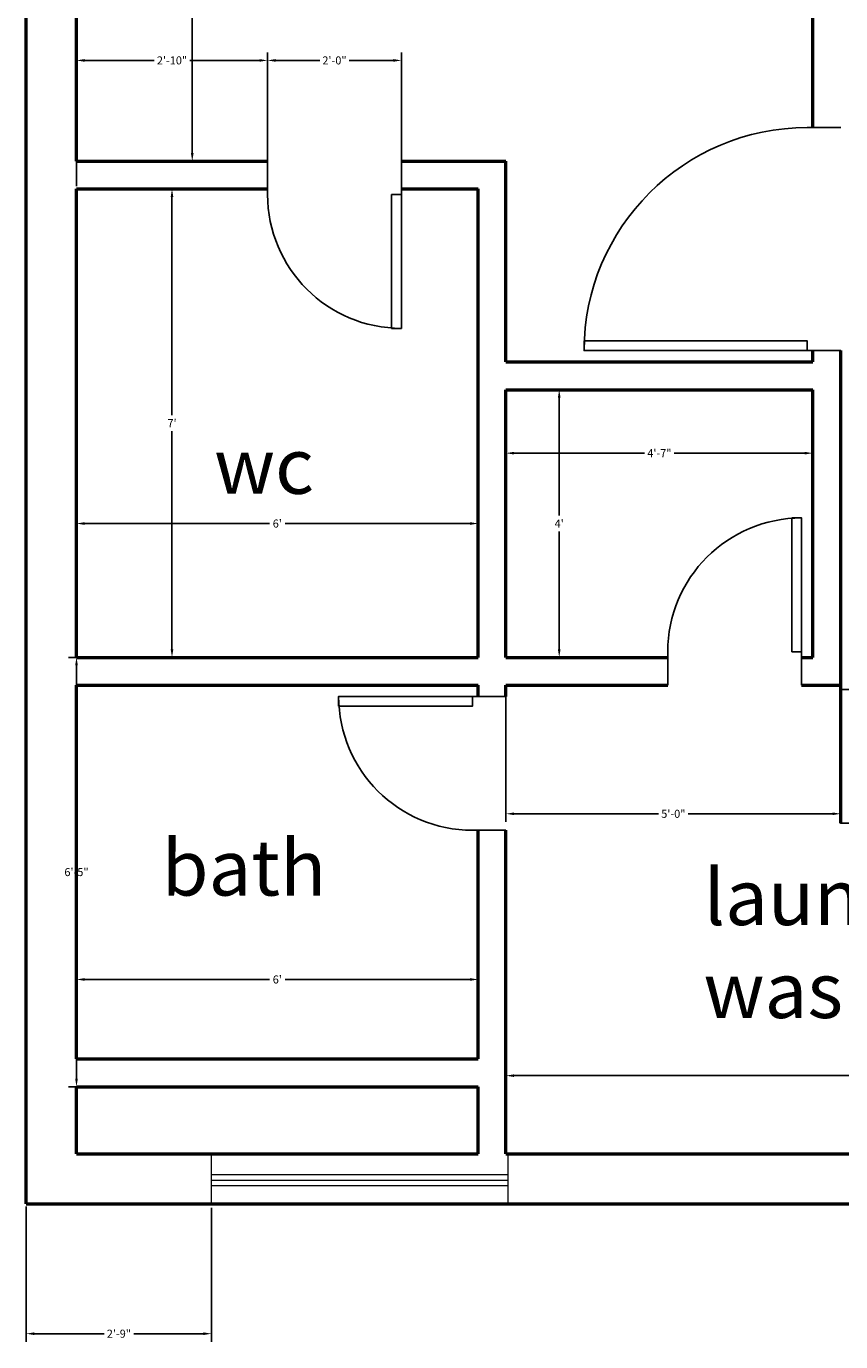
# Model space of a CAD drawing. Units: inches. Extents: x 325 to 804, y 366 to 834.
# Tile 1 of 6: x 350 to 496, y 367 to 603. Entities that reach past the tile are written whole.
import ezdxf

# ---------------------------------------------------------------- set-up
doc = ezdxf.new("R2010")
doc.units = ezdxf.units.IN
doc.header["$MEASUREMENT"] = 0
doc.layers.get('0').update_dxf_attribs({"color": 4})
for name, color, linetype, lineweight in [('A-ANNO-DIMS', 2, 'Continuous', 18), ('A-AREA-IDEN', 7, 'Continuous', 25), ('A-WALL', 7, 'Continuous', 50), ('door', 10, 'Continuous', 25), ('window', 3, 'Continuous', 18)]:
    doc.layers.add(name, color=color, linetype=linetype, lineweight=lineweight)
doc.styles.get("Standard").update_dxf_attribs({"font": 'arial.ttf'})
doc.dimstyles.get("Standard").update_dxf_attribs({"dimscale": 8, "dimtxt": 0.18, "dimasz": 0.18, "dimexe": 0.18, "dimexo": 0.0625, "dimgap": 0.09, "dimtad": 0, "dimtih": 1, "dimtoh": 1, "dimdec": 0, "dimzin": 0, "dimdsep": 46, "dimlunit": 3, "dimtxsty": 'Standard', "dimcen": 0.09, "dimadec": 0, "dimazin": 0, "dimtfac": 1, "dimtdec": 0, "dimtofl": 0, "dimtmove": 0, "dimatfit": 3, "dimfxl": 1, "dimtolj": 1, "dimtzin": 0, "dimarcsym": 0})

# ---------------------------------------------------------------- blocks, each defined once
blk = doc.blocks.new('*U3')
for p, q in [((0, 0), (0, -6)), ((40, 0), (40, -6))]:
    blk.add_line(p, q)
blk.add_lwpolyline([(0, 0), (0, 40), (1.75, 40), (1.75, 0)], close=True)
blk.add_arc((0, 0), 40, 0, 90)
blk = doc.blocks.new('*U4')
for p, q in [((0, 0), (0, -6)), ((-24, 0), (-24, -6))]:
    blk.add_line(p, q)
blk.add_lwpolyline([(0, 0), (0, 24), (-1.75, 24), (-1.75, 0)], close=True)
blk.add_arc((0, 0), 24, 90, 180)
blk = doc.blocks.new('*U5')
for p, q in [((-24, 0), (-24, 6)), ((0, 0), (0, 6))]:
    blk.add_line(p, q)
blk.add_lwpolyline([(0, 0), (0, -24), (-1.75, -24), (-1.75, 0)], close=True)
blk.add_arc((0, 0), 24, 180, 270)
blk = doc.blocks.new('*U6')
for p, q in [((-24, 0), (-24, 6)), ((0, 0), (0, 6))]:
    blk.add_line(p, q)
blk.add_lwpolyline([(0, 0), (0, -24), (-1.75, -24), (-1.75, 0)], close=True)
blk.add_arc((0, 0), 24, 180, 270)
blk = doc.blocks.new('*U7')
for p, q in [((0, 0), (0, -6)), ((-24, 0), (-24, -6))]:
    blk.add_line(p, q)
blk.add_lwpolyline([(0, 0), (0, 24), (-1.75, 24), (-1.75, 0)], close=True)
blk.add_arc((0, 0), 24, 90, 180)
blk = doc.blocks.new('*D9')
at = {"layer": 'A-ANNO-DIMS', "color": 0, "lineweight": -2, "transparency": 16777216}
for p, q in [((359.97, 752.54), (381.66, 752.54)), ((380.22, 751.1), (380.22, 674.43)), ((380.22, 579.98), (380.22, 656.65)), ((359.97, 578.54), (381.66, 578.54))]:
    blk.add_line(p, q, dxfattribs=at)
at = {"layer": 'A-ANNO-DIMS', "color": 0, "transparency": 16777216}
for points in [[(379.98, 751.1), (380.46, 751.1), (380.22, 752.54)], [(379.98, 579.98), (380.46, 579.98), (380.22, 578.54)]]:
    blk.add_solid(points, dxfattribs=at)
at = {"layer": 'Defpoints', "color": 0, "transparency": 16777216}
for p in [(359.47, 752.54), (359.47, 578.54), (380.22, 578.54)]:
    blk.add_point(p, dxfattribs=at)
at = {"layer": 'A-ANNO-DIMS', "color": 0, "transparency": 16777216, "insert": (380.22, 665.54), "char_height": 1.44, "attachment_point": 5}
blk.add_mtext('\\A1;{\\H11.11111x;14\'-6"}', dxfattribs=at)
blk = doc.blocks.new('*D13')
at = {"layer": 'A-ANNO-DIMS', "color": 0, "lineweight": -2, "transparency": 16777216}
for p, q in [((377.09, 573.54), (378.03, 573.54)), ((376.59, 572.1), (376.59, 532.98)), ((376.59, 490.98), (376.59, 530.1)), ((377.09, 489.54), (378.03, 489.54))]:
    blk.add_line(p, q, dxfattribs=at)
at = {"layer": 'A-ANNO-DIMS', "color": 0, "transparency": 16777216}
for points in [[(376.35, 572.1), (376.83, 572.1), (376.59, 573.54)], [(376.35, 490.98), (376.83, 490.98), (376.59, 489.54)]]:
    blk.add_solid(points, dxfattribs=at)
at = {"layer": 'Defpoints', "color": 0, "transparency": 16777216}
for p in [(376.59, 573.54), (376.59, 489.54), (376.59, 489.54)]:
    blk.add_point(p, dxfattribs=at)
at = {"layer": 'A-ANNO-DIMS', "color": 0, "transparency": 16777216, "insert": (376.59, 531.54), "char_height": 1.44, "attachment_point": 5}
blk.add_mtext("\\A1;7'", dxfattribs=at)
blk = doc.blocks.new('*D14')
at = {"layer": 'A-ANNO-DIMS', "color": 0, "lineweight": -2, "transparency": 16777216}
for p, q in [((359.47, 508.32), (359.47, 514.98)), ((431.47, 508.32), (431.47, 514.98)), ((360.91, 513.54), (394.09, 513.54)), ((430.03, 513.54), (396.86, 513.54))]:
    blk.add_line(p, q, dxfattribs=at)
at = {"layer": 'A-ANNO-DIMS', "color": 0, "transparency": 16777216}
for points in [[(360.91, 513.78), (360.91, 513.3), (359.47, 513.54)], [(430.03, 513.78), (430.03, 513.3), (431.47, 513.54)]]:
    blk.add_solid(points, dxfattribs=at)
at = {"layer": 'Defpoints', "color": 0, "transparency": 16777216}
for p in [(431.47, 513.54), (359.47, 507.82), (431.47, 507.82)]:
    blk.add_point(p, dxfattribs=at)
at = {"layer": 'A-ANNO-DIMS', "color": 0, "transparency": 16777216, "insert": (395.47, 513.54), "char_height": 1.44, "attachment_point": 5}
blk.add_mtext("\\A1;6'", dxfattribs=at)
blk = doc.blocks.new('*D15')
at = {"layer": 'A-ANNO-DIMS', "color": 0, "lineweight": -2, "transparency": 16777216}
for p, q in [((376.09, 489.54), (358.03, 489.54)), ((359.47, 488.1), (359.47, 452.49)), ((359.47, 413.98), (359.47, 449.58)), ((376.09, 412.54), (358.03, 412.54))]:
    blk.add_line(p, q, dxfattribs=at)
at = {"layer": 'A-ANNO-DIMS', "color": 0, "transparency": 16777216}
for points in [[(359.23, 488.1), (359.71, 488.1), (359.47, 489.54)], [(359.23, 413.98), (359.71, 413.98), (359.47, 412.54)]]:
    blk.add_solid(points, dxfattribs=at)
at = {"layer": 'Defpoints', "color": 0, "transparency": 16777216}
for p in [(376.59, 489.54), (359.47, 412.54), (376.59, 412.54)]:
    blk.add_point(p, dxfattribs=at)
at = {"layer": 'A-ANNO-DIMS', "color": 0, "transparency": 16777216, "insert": (359.47, 451.04), "char_height": 1.44, "attachment_point": 5}
blk.add_mtext('\\A1;6\'-5"', dxfattribs=at)
blk = doc.blocks.new('*D16')
at = {"layer": 'A-ANNO-DIMS', "color": 0, "lineweight": -2, "transparency": 16777216}
for p, q in [((359.47, 432.28), (359.47, 433.22)), ((360.91, 431.78), (394.09, 431.78)), ((430.03, 431.78), (396.86, 431.78)), ((431.47, 432.28), (431.47, 433.22))]:
    blk.add_line(p, q, dxfattribs=at)
at = {"layer": 'A-ANNO-DIMS', "color": 0, "transparency": 16777216}
for points in [[(360.91, 432.02), (360.91, 431.54), (359.47, 431.78)], [(430.03, 432.02), (430.03, 431.54), (431.47, 431.78)]]:
    blk.add_solid(points, dxfattribs=at)
at = {"layer": 'Defpoints', "color": 0, "transparency": 16777216}
for p in [(359.47, 431.78), (431.47, 431.78), (431.47, 431.78)]:
    blk.add_point(p, dxfattribs=at)
at = {"layer": 'A-ANNO-DIMS', "color": 0, "transparency": 16777216, "insert": (395.47, 431.78), "char_height": 1.44, "attachment_point": 5}
blk.add_mtext("\\A1;6'", dxfattribs=at)
blk = doc.blocks.new('*D17')
at = {"layer": 'A-ANNO-DIMS', "color": 0, "lineweight": -2, "transparency": 16777216}
for p, q in [((436.47, 417.88), (436.47, 413.09)), ((580.47, 417.88), (580.47, 413.09)), ((437.91, 414.53), (506.6, 414.53)), ((579.03, 414.53), (510.35, 414.53))]:
    blk.add_line(p, q, dxfattribs=at)
at = {"layer": 'A-ANNO-DIMS', "color": 0, "transparency": 16777216}
for points in [[(437.91, 414.77), (437.91, 414.29), (436.47, 414.53)], [(579.03, 414.77), (579.03, 414.29), (580.47, 414.53)]]:
    blk.add_solid(points, dxfattribs=at)
at = {"layer": 'Defpoints', "color": 0, "transparency": 16777216}
for p in [(436.47, 418.38), (580.47, 418.38), (580.47, 414.53)]:
    blk.add_point(p, dxfattribs=at)
at = {"layer": 'A-ANNO-DIMS', "color": 0, "transparency": 16777216, "insert": (508.47, 414.53), "char_height": 1.44, "attachment_point": 5}
blk.add_mtext("\\A1;12'", dxfattribs=at)
blk = doc.blocks.new('*D23')
at = {"layer": 'A-ANNO-DIMS', "color": 0, "lineweight": -2, "transparency": 16777216}
for p, q in [((436.47, 537.04), (436.47, 524.72)), ((491.47, 537.04), (491.47, 524.72)), ((437.91, 526.16), (461.31, 526.16)), ((490.03, 526.16), (466.64, 526.16))]:
    blk.add_line(p, q, dxfattribs=at)
at = {"layer": 'A-ANNO-DIMS', "color": 0, "transparency": 16777216}
for points in [[(437.91, 526.4), (437.91, 525.92), (436.47, 526.16)], [(490.03, 526.4), (490.03, 525.92), (491.47, 526.16)]]:
    blk.add_solid(points, dxfattribs=at)
at = {"layer": 'Defpoints', "color": 0, "transparency": 16777216}
for p in [(436.47, 537.54), (491.47, 537.54), (491.47, 526.16)]:
    blk.add_point(p, dxfattribs=at)
at = {"layer": 'A-ANNO-DIMS', "color": 0, "transparency": 16777216, "insert": (463.97, 526.16), "char_height": 1.44, "attachment_point": 5}
blk.add_mtext('\\A1;4\'-7"', dxfattribs=at)
blk = doc.blocks.new('*D24')
at = {"layer": 'A-ANNO-DIMS', "color": 0, "lineweight": -2, "transparency": 16777216}
for p, q in [((446.01, 536.1), (446.01, 514.98)), ((446.51, 537.54), (447.45, 537.54)), ((446.01, 490.98), (446.01, 512.1)), ((446.51, 489.54), (447.45, 489.54))]:
    blk.add_line(p, q, dxfattribs=at)
at = {"layer": 'A-ANNO-DIMS', "color": 0, "transparency": 16777216}
for points in [[(445.77, 536.1), (446.25, 536.1), (446.01, 537.54)], [(445.77, 490.98), (446.25, 490.98), (446.01, 489.54)]]:
    blk.add_solid(points, dxfattribs=at)
at = {"layer": 'Defpoints', "color": 0, "transparency": 16777216}
for p in [(446.01, 537.54), (446.01, 489.54), (446.01, 489.54)]:
    blk.add_point(p, dxfattribs=at)
at = {"layer": 'A-ANNO-DIMS', "color": 0, "transparency": 16777216, "insert": (446.01, 513.54), "char_height": 1.44, "attachment_point": 5}
blk.add_mtext("\\A1;4'", dxfattribs=at)
blk = doc.blocks.new('*D41')
at = {"layer": 'A-ANNO-DIMS', "color": 0, "lineweight": -2, "transparency": 16777216}
for p, q in [((393.72, 574.04), (393.72, 598.03)), ((417.72, 574.04), (417.72, 598.03)), ((395.16, 596.59), (403.07, 596.59)), ((416.28, 596.59), (408.36, 596.59))]:
    blk.add_line(p, q, dxfattribs=at)
at = {"layer": 'A-ANNO-DIMS', "color": 0, "transparency": 16777216}
for points in [[(395.16, 596.83), (395.16, 596.35), (393.72, 596.59)], [(416.28, 596.83), (416.28, 596.35), (417.72, 596.59)]]:
    blk.add_solid(points, dxfattribs=at)
at = {"layer": 'Defpoints', "color": 0, "transparency": 16777216}
for p in [(417.72, 596.59), (393.72, 573.54), (417.72, 573.54)]:
    blk.add_point(p, dxfattribs=at)
at = {"layer": 'A-ANNO-DIMS', "color": 0, "transparency": 16777216, "insert": (405.72, 596.59), "char_height": 1.44, "attachment_point": 5}
blk.add_mtext('\\A1;2\'-0"', dxfattribs=at)
blk = doc.blocks.new('*D45')
at = {"layer": 'A-ANNO-DIMS', "color": 0, "lineweight": -2, "transparency": 16777216}
for p, q in [((359.47, 574.04), (359.47, 598.03)), ((393.72, 574.04), (393.72, 598.03)), ((360.91, 596.59), (373.39, 596.59)), ((392.28, 596.59), (379.8, 596.59))]:
    blk.add_line(p, q, dxfattribs=at)
at = {"layer": 'A-ANNO-DIMS', "color": 0, "transparency": 16777216}
for points in [[(360.91, 596.83), (360.91, 596.35), (359.47, 596.59)], [(392.28, 596.83), (392.28, 596.35), (393.72, 596.59)]]:
    blk.add_solid(points, dxfattribs=at)
at = {"layer": 'Defpoints', "color": 0, "transparency": 16777216}
for p in [(393.72, 596.59), (359.47, 573.54), (393.72, 573.54)]:
    blk.add_point(p, dxfattribs=at)
at = {"layer": 'A-ANNO-DIMS', "color": 0, "transparency": 16777216, "insert": (376.59, 596.59), "char_height": 1.44, "attachment_point": 5}
blk.add_mtext('\\A1;2\'-10"', dxfattribs=at)
blk = doc.blocks.new('*D46')
at = {"layer": 'A-ANNO-DIMS', "color": 0, "lineweight": -2, "transparency": 16777216}
for p, q in [((436.47, 484.04), (436.47, 460.05)), ((496.47, 484.04), (496.47, 460.05)), ((437.91, 461.49), (463.84, 461.49)), ((495.03, 461.49), (469.11, 461.49))]:
    blk.add_line(p, q, dxfattribs=at)
at = {"layer": 'A-ANNO-DIMS', "color": 0, "transparency": 16777216}
for points in [[(437.91, 461.73), (437.91, 461.25), (436.47, 461.49)], [(495.03, 461.73), (495.03, 461.25), (496.47, 461.49)]]:
    blk.add_solid(points, dxfattribs=at)
at = {"layer": 'Defpoints', "color": 0, "transparency": 16777216}
for p in [(436.47, 484.54), (496.47, 484.54), (436.47, 461.49)]:
    blk.add_point(p, dxfattribs=at)
at = {"layer": 'A-ANNO-DIMS', "color": 0, "transparency": 16777216, "insert": (466.47, 461.49), "char_height": 1.44, "attachment_point": 5}
blk.add_mtext('\\A1;5\'-0"', dxfattribs=at)
blk = doc.blocks.new('*D48')
at = {"layer": 'A-ANNO-DIMS', "color": 0, "lineweight": -2, "transparency": 16777216}
for p, q in [((350.47, 391.04), (350.47, 366.82)), ((383.67, 390.81), (383.67, 366.82)), ((351.91, 368.26), (364.42, 368.26)), ((382.23, 368.26), (369.72, 368.26))]:
    blk.add_line(p, q, dxfattribs=at)
at = {"layer": 'A-ANNO-DIMS', "color": 0, "transparency": 16777216}
for points in [[(351.91, 368.5), (351.91, 368.02), (350.47, 368.26)], [(382.23, 368.5), (382.23, 368.02), (383.67, 368.26)]]:
    blk.add_solid(points, dxfattribs=at)
at = {"layer": 'Defpoints', "color": 0, "transparency": 16777216}
for p in [(350.47, 391.54), (383.67, 391.31), (383.67, 368.26)]:
    blk.add_point(p, dxfattribs=at)
at = {"layer": 'A-ANNO-DIMS', "color": 0, "transparency": 16777216, "insert": (367.07, 368.26), "char_height": 1.44, "attachment_point": 5}
blk.add_mtext('\\A1;2\'-9"', dxfattribs=at)

msp = doc.modelspace()

# ---------------------------------------------------------------- linework, layer by layer
at = {"layer": 'A-WALL'}
for p, q in [((350.47, 391.54), (350.47, 761.54)), ((359.47, 578.54), (359.47, 752.54)), ((491.47, 584.54), (491.47, 752.54)), ((359.47, 578.54), (393.72, 578.54)), ((417.72, 578.54), (436.47, 578.54)), ((436.47, 542.54), (436.47, 578.54)), ((359.47, 573.54), (393.72, 573.54)), ((359.47, 489.54), (359.47, 573.54)), ((417.72, 573.54), (431.47, 573.54)), ((431.47, 489.54), (431.47, 573.54)), ((436.47, 542.54), (491.47, 542.54)), ((491.47, 542.54), (491.47, 544.54)), ((496.47, 459.78), (496.47, 544.54)), ((436.47, 489.54), (436.47, 537.54)), ((436.47, 537.54), (491.47, 537.54)), ((491.47, 489.54), (491.47, 537.54)), ((359.47, 489.54), (431.47, 489.54)), ((436.47, 489.54), (465.47, 489.54)), ((489.47, 489.54), (491.47, 489.54)), ((359.47, 484.54), (431.47, 484.54)), ((359.47, 417.54), (359.47, 484.54)), ((431.47, 482.54), (431.47, 484.54)), ((436.47, 484.54), (465.47, 484.54)), ((436.47, 482.54), (436.47, 484.54)), ((489.47, 484.54), (496.47, 484.54)), ((431.47, 417.54), (431.47, 458.54)), ((436.47, 400.54), (436.47, 458.54)), ((359.47, 417.54), (431.47, 417.54)), ((359.47, 400.54), (359.47, 412.54)), ((359.47, 412.54), (431.47, 412.54)), ((431.47, 400.54), (431.47, 412.54)), ((359.47, 400.54), (431.47, 400.54)), ((436.47, 400.54), (580.47, 400.54)), ((350.47, 391.54), (774.47, 391.54))]:
    msp.add_line(p, q, dxfattribs=at)
at = {"layer": 'door'}
for p, q in [((417.72, 578.54), (417.72, 573.54)), ((491.47, 544.54), (496.47, 544.54)), ((489.47, 489.54), (489.47, 484.54)), ((436.47, 482.54), (431.47, 482.54))]:
    msp.add_line(p, q, dxfattribs=at)
at = {"layer": 'window'}
for p, q in [((383.67, 396.81), (436.81, 396.81)), ((383.67, 395.81), (436.81, 395.81)), ((383.67, 394.81), (436.81, 394.81))]:
    msp.add_line(p, q, dxfattribs=at)
msp.add_lwpolyline([(436.81, 400.31), (436.81, 391.31), (383.67, 391.31), (383.67, 400.31)], dxfattribs=at)

# ---------------------------------------------------------------- block references
at = {"layer": 'door', "rotation": 90}
for name, p in [('*U3', (490.47, 544.54)), ('*U7', (430.47, 482.54))]:
    msp.add_blockref(name, p, dxfattribs=at)
at = {"layer": 'door'}
for name, p in [('*U5', (417.72, 572.54)), ('*U4', (489.47, 490.54))]:
    msp.add_blockref(name, p, dxfattribs=at)
at = {"layer": 'door', "xscale": -1}
msp.add_blockref('*U6', (496.47, 483.78), dxfattribs=at)

# ---------------------------------------------------------------- texts
at = {"layer": 'A-AREA-IDEN', "char_height": 10, "attachment_point": 1}
for s, width, heights, insert in [('wc', 25.6907, [0], (384.13, 528.87)), ('bath', 20.8578, [0.203], (374.71, 456.83)), ('laundry washer/dryer', 25.6907, [0], (471.88, 451.54))]:
    msp.add_mtext_dynamic_manual_height_columns(s, width=width, gutter_width=1, heights=heights, dxfattribs=dict(at, insert=insert))

# ---------------------------------------------------------------- dimensions: what is measured, and where the dimension line sits
at = {"layer": 'A-ANNO-DIMS'}
dim = msp.add_linear_dim(base=(380.22, 578.54), p1=(359.47, 752.54), p2=(359.47, 578.54), angle=90, text='{\\H11.11111x;<>}', dimstyle='Standard', override={"dimclrd": 0, "dimclre": 0, "dimclrt": 0}, dxfattribs=at)
dim.commit()
dim.dimension.update_dxf_attribs({"geometry": '*D9', "text_midpoint": (380.22, 665.54)})
for base, p1, p2, override, picture, middle in [((393.717, 596.5889), (359.4724, 573.5389), (393.717, 573.5389), {"dimdec": 1, "dimlfac": 1, "dimrnd": 0, "dimzin": 1, "dimdsep": 46, "dimlunit": 4, "dimfrac": 2}, '*D45', (376.5947, 596.5889)), ((417.72, 596.59), (393.72, 573.54), (417.72, 573.54), {"dimdec": 1, "dimlfac": 1, "dimrnd": 0, "dimzin": 1, "dimdsep": 46, "dimlunit": 4, "dimfrac": 2}, '*D41', (405.72, 596.59)), ((491.47, 526.16), (436.47, 537.54), (491.47, 537.54), {"dimclrd": 0, "dimclre": 0, "dimclrt": 0}, '*D23', (463.97, 526.16)), ((431.47, 513.54), (359.47, 507.82), (431.47, 507.82), {"dimclrd": 0, "dimclre": 0, "dimclrt": 0}, '*D14', (395.47, 513.54)), ((431.47, 431.78), (359.47, 431.78), (431.47, 431.78), {"dimclrd": 0, "dimclre": 0, "dimclrt": 0}, '*D16', (395.47, 431.78)), ((580.47, 414.53), (436.47, 418.38), (580.47, 418.38), {"dimclrd": 0, "dimclre": 0, "dimclrt": 0}, '*D17', (508.47, 414.53)), ((383.67, 368.26), (350.47, 391.54), (383.67, 391.31), {"dimdec": 1, "dimlfac": 1, "dimrnd": 0, "dimzin": 1, "dimdsep": 46, "dimlunit": 4, "dimfrac": 2}, '*D48', (367.07, 368.26))]:
    dim = msp.add_linear_dim(base=base, p1=p1, p2=p2, dimstyle='Standard', override=override, dxfattribs=at)
    dim.commit()
    dim.dimension.update_dxf_attribs({"geometry": picture, "text_midpoint": middle})
for base, p1, p2, angle, override, picture, middle in [((376.59, 489.54), (376.59, 573.54), (376.59, 489.54), 90, {"dimclrd": 0, "dimclre": 0, "dimclrt": 0}, '*D13', (376.59, 531.54)), ((446.01, 489.54), (446.01, 537.54), (446.01, 489.54), 90, {"dimclrd": 0, "dimclre": 0, "dimclrt": 0}, '*D24', (446.01, 513.54)), ((359.47, 412.54), (376.59, 489.54), (376.59, 412.54), 90, {"dimclrd": 0, "dimclre": 0, "dimclrt": 0}, '*D15', (359.47, 451.04)), ((436.47, 461.49), (496.47, 484.54), (436.47, 484.54), 180, {"dimdec": 1, "dimlfac": 1, "dimrnd": 0, "dimzin": 1, "dimdsep": 46, "dimlunit": 4, "dimfrac": 2}, '*D46', (466.47, 461.49))]:
    dim = msp.add_linear_dim(base=base, p1=p1, p2=p2, angle=angle, dimstyle='Standard', override=override, dxfattribs=at)
    dim.commit()
    dim.dimension.update_dxf_attribs({"geometry": picture, "text_midpoint": middle})

doc.saveas('drawing.dxf')
